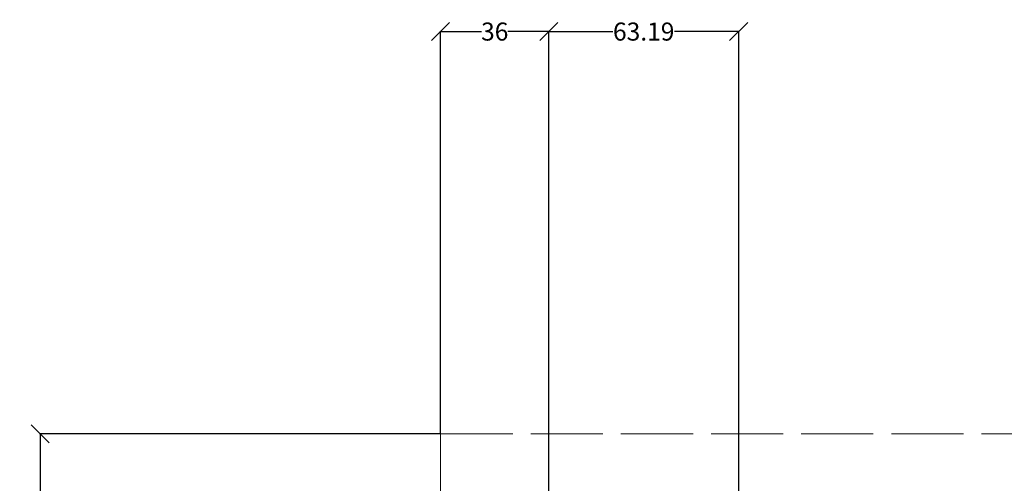
# Model space of a CAD drawing. Units: inches. Extents: x -1198 to -69, y -512 to 437.
# Tile 18 of 50: x -1195 to -867, y 283 to 437. Entities that reach past the tile are written whole.
import ezdxf

# ---------------------------------------------------------------- set-up
doc = ezdxf.new("R2010")
doc.units = ezdxf.units.IN
doc.header["$MEASUREMENT"] = 0
doc.linetypes.add('ACAD_ISO02W100', pattern=[15, 12, -3])
doc.layers.add('A-ANNO-DIMS', color=2, linetype='Continuous', lineweight=18)
doc.layers.add('C-PROP', color=141, linetype='ACAD_ISO02W100', lineweight=18)
doc.styles.get("Standard").update_dxf_attribs({"font": 'arial.ttf'})
doc.dimstyles.get("Standard").update_dxf_attribs({"dimtxt": 6, "dimasz": 6, "dimexe": 0.18, "dimexo": 0.0625, "dimgap": 0.09, "dimtad": 0, "dimtih": 1, "dimtoh": 1, "dimdec": 0, "dimzin": 0, "dimdsep": 46, "dimlunit": 4, "dimtxsty": 'Standard', "dimblk": 'OBLIQUE', "dimcen": 0.09, "dimadec": 0, "dimazin": 0, "dimtfac": 1, "dimtdec": 0, "dimtofl": 0, "dimtmove": 0, "dimatfit": 3, "dimfxl": 1, "dimtolj": 1, "dimtzin": 0, "dimarcsym": 0})

# ---------------------------------------------------------------- blocks, each defined once
blk = doc.blocks.new('_Oblique')
at = {"color": 0, "linetype": 'ByBlock', "lineweight": -2}
blk.add_line((-0.5, -0.5), (0.5, 0.5), dxfattribs=at)
blk = doc.blocks.new('*D61')
at = {"layer": 'A-ANNO-DIMS', "color": 0, "lineweight": -2, "ltscale": 10, "transparency": 16777216}
for p, q in [((-1054.81, 299.23), (-1188.2, 299.23)), ((-1188.02, 299.23), (-1188.02, 20.38)), ((-1188.02, -264.77), (-1188.02, 14.07)), ((-1054.81, -264.77), (-1188.2, -264.77))]:
    blk.add_line(p, q, dxfattribs=at)
at = {"layer": 'DEFPOINTS', "color": 0, "ltscale": 10, "transparency": 16777216}
for p in [(-1054.75, 299.23), (-1188.02, -264.77), (-1054.75, -264.77)]:
    blk.add_point(p, dxfattribs=at)
at = {"layer": 'A-ANNO-DIMS', "color": 0, "lineweight": -2, "ltscale": 10, "transparency": 16777216, "xscale": 6, "yscale": 6, "zscale": 6}
for p, rotation in [((-1188.02, 299.23), 90), ((-1188.02, -264.77), 270)]:
    blk.add_blockref('_Oblique', p, dxfattribs=dict(at, rotation=rotation))
at = {"layer": 'A-ANNO-DIMS', "color": 0, "ltscale": 10, "transparency": 16777216, "insert": (-1188.02, 17.23), "char_height": 6, "attachment_point": 5}
blk.add_mtext('\\A1;564', dxfattribs=at)
blk = doc.blocks.new('*D65')
at = {"layer": 'A-ANNO-DIMS', "color": 0, "lineweight": -2, "ltscale": 10, "transparency": 16777216}
for p, q in [((-1054.75, 299.29), (-1054.75, 433.18)), ((-1054.75, 433), (-1041.13, 433)), ((-1018.75, 433), (-1032.37, 433)), ((-1018.75, 263.29), (-1018.75, 433.18))]:
    blk.add_line(p, q, dxfattribs=at)
at = {"layer": 'DEFPOINTS', "color": 0, "ltscale": 10, "transparency": 16777216}
for p in [(-1018.75, 433), (-1054.75, 299.23), (-1018.75, 263.23)]:
    blk.add_point(p, dxfattribs=at)
at = {"layer": 'A-ANNO-DIMS', "color": 0, "lineweight": -2, "ltscale": 10, "transparency": 16777216, "xscale": 6, "yscale": 6, "zscale": 6, "rotation": 180}
blk.add_blockref('_Oblique', (-1054.75, 433), dxfattribs=at)
at = {"layer": 'A-ANNO-DIMS', "color": 0, "lineweight": -2, "ltscale": 10, "transparency": 16777216, "xscale": 6, "yscale": 6, "zscale": 6}
blk.add_blockref('_Oblique', (-1018.75, 433), dxfattribs=at)
at = {"layer": 'A-ANNO-DIMS', "color": 0, "ltscale": 10, "transparency": 16777216, "insert": (-1036.75, 433), "char_height": 6, "attachment_point": 5}
blk.add_mtext('\\A1;36', dxfattribs=at)
blk = doc.blocks.new('*D78')
at = {"layer": 'A-ANNO-DIMS', "color": 0, "lineweight": -2, "ltscale": 10, "transparency": 16777216}
for p, q in [((-1018.75, 263.29), (-1018.75, 433.18)), ((-1018.75, 433), (-997.39, 433)), ((-955.56, 433), (-976.92, 433)), ((-955.56, 263.29), (-955.56, 433.18))]:
    blk.add_line(p, q, dxfattribs=at)
at = {"layer": 'DEFPOINTS', "color": 0, "ltscale": 10, "transparency": 16777216}
for p in [(-955.56, 433), (-1018.75, 263.23), (-955.56, 263.23)]:
    blk.add_point(p, dxfattribs=at)
at = {"layer": 'A-ANNO-DIMS', "color": 0, "lineweight": -2, "ltscale": 10, "transparency": 16777216, "xscale": 6, "yscale": 6, "zscale": 6, "rotation": 180}
blk.add_blockref('_Oblique', (-1018.75, 433), dxfattribs=at)
at = {"layer": 'A-ANNO-DIMS', "color": 0, "lineweight": -2, "ltscale": 10, "transparency": 16777216, "xscale": 6, "yscale": 6, "zscale": 6}
blk.add_blockref('_Oblique', (-955.56, 433), dxfattribs=at)
at = {"layer": 'A-ANNO-DIMS', "color": 0, "ltscale": 10, "transparency": 16777216, "insert": (-987.16, 433), "char_height": 6, "attachment_point": 5}
blk.add_mtext('\\A1;63.19', dxfattribs=at)

msp = doc.modelspace()

# ---------------------------------------------------------------- linework, layer by layer
at = {"layer": 'C-PROP', "ltscale": 2}
msp.add_lwpolyline([(-1054.7509, 299.2277), (-334.7509, 299.2277), (-334.7509, -264.7723), (-1054.7509, -264.7723)], close=True, dxfattribs=at)

# ---------------------------------------------------------------- dimensions: what is measured, and where the dimension line sits
at = {"layer": 'A-ANNO-DIMS', "ltscale": 10}
for base, p1, p2, override, picture, middle in [((-1018.7509, 433.0036), (-1054.7509, 299.2277), (-1018.7509, 263.2277), {"dimdec": 0, "dimlfac": 1, "dimrnd": 0, "dimzin": 0, "dimdsep": 46, "dimlunit": 2}, '*D65', (-1036.7509, 433.0036)), ((-955.5591, 433.0036), (-1018.7509, 263.2277), (-955.5591, 263.2277), {"dimdec": 2, "dimlfac": 1, "dimrnd": 0, "dimzin": 0, "dimdsep": 46, "dimlunit": 2}, '*D78', (-987.155, 433.0036))]:
    dim = msp.add_linear_dim(base=base, p1=p1, p2=p2, dimstyle='Standard', override=override, dxfattribs=at)
    dim.commit()
    dim.dimension.update_dxf_attribs({"geometry": picture, "text_midpoint": middle})
dim = msp.add_linear_dim(base=(-1188.0248, -264.7723), p1=(-1054.7509, 299.2277), p2=(-1054.7509, -264.7723), angle=90, dimstyle='Standard', override={"dimdec": 0, "dimlfac": 1, "dimrnd": 0, "dimzin": 0, "dimdsep": 46, "dimlunit": 2}, dxfattribs=at)
dim.commit()
dim.dimension.update_dxf_attribs({"geometry": '*D61', "text_midpoint": (-1188.0248, 17.2277)})

doc.saveas('drawing.dxf')
